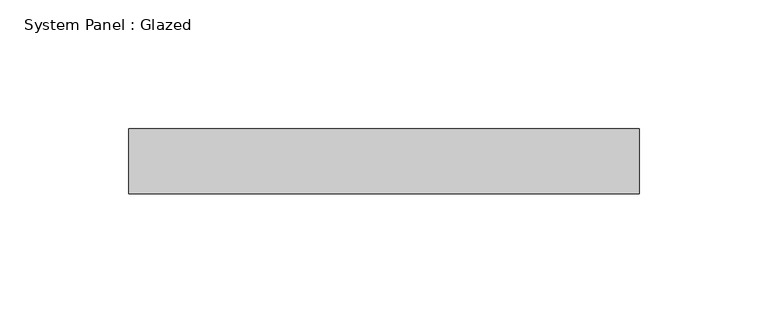
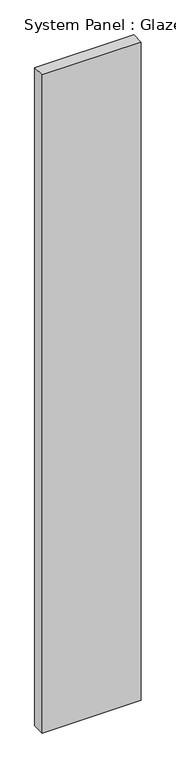
"""IFC4 building model written with IfcOpenShell, lengths in millimetres: plate geometry, System Panel : Glazed."""

from ifc_helpers import new_model, si_unit, origin, origin_with_axes, place, context, project, spatial, polyline, outline, extrude, source, transform, mapped, element, save


def system_panel_glazed_ccd8c114(model_context):
    return source(origin(), model_context, "Body", "SweptSolid", [
        extrude(outline(polyline([(99.3775, 19.05), (-99.3775, 19.05), (-99.3775, 44.45), (99.3775, 44.45), (99.3775, 19.05)])), origin_with_axes(), (0.0, 0.0, 1.0), 1395.1131867),
    ])


if __name__ == "__main__":
    model = new_model("IFC4")
    model_context = context("Model", 3, world=origin())
    ifc_project = project(units=[si_unit("LENGTHUNIT", "METRE", prefix="MILLI")], contexts=[model_context])
    site = spatial("IfcSite", under=ifc_project)
    building = spatial("IfcBuilding", under=site)
    placement = place(None, origin())
    system_panel_glazed_shape = system_panel_glazed_ccd8c114(model_context)
    element("IfcPlate", 1, ObjectType="System Panel : Glazed", at=placement, inside=building, context=model_context, shape_type="MappedRepresentation", body=[
        mapped(system_panel_glazed_shape, transform((0.0, 0.0, 0.0), x_axis=(1.0, 0.0, 0.0), y_axis=(0.0, 1.0, 0.0), z_axis=(0.0, 0.0, 1.0))),
    ])
    save(model, "model.ifc")

# Revit data of these elements
# Type "System Panel : Glazed"
#   Construction Type Id = "GSP4R"
#   Analytic Construction = "1/8 in Pilkington single glazing"
#   Visual Light Transmittance = 0.9
#   Solar Heat Gain Coefficient = 0.86
#   Heat Transfer Coefficient (U) = 1.18115 BTU/(h·ft²·°F)
#   Define Thermal Properties by = 1
# Element 1 (IfcPlate, "System Panel : Glazed")
#   Materials on its faces: "Glass"
# Materials
#   "Glass": class "Glass", colour RGB 0 128 192, transparency 0.75, Description = "Soda Lime Glass", Cost = 0
